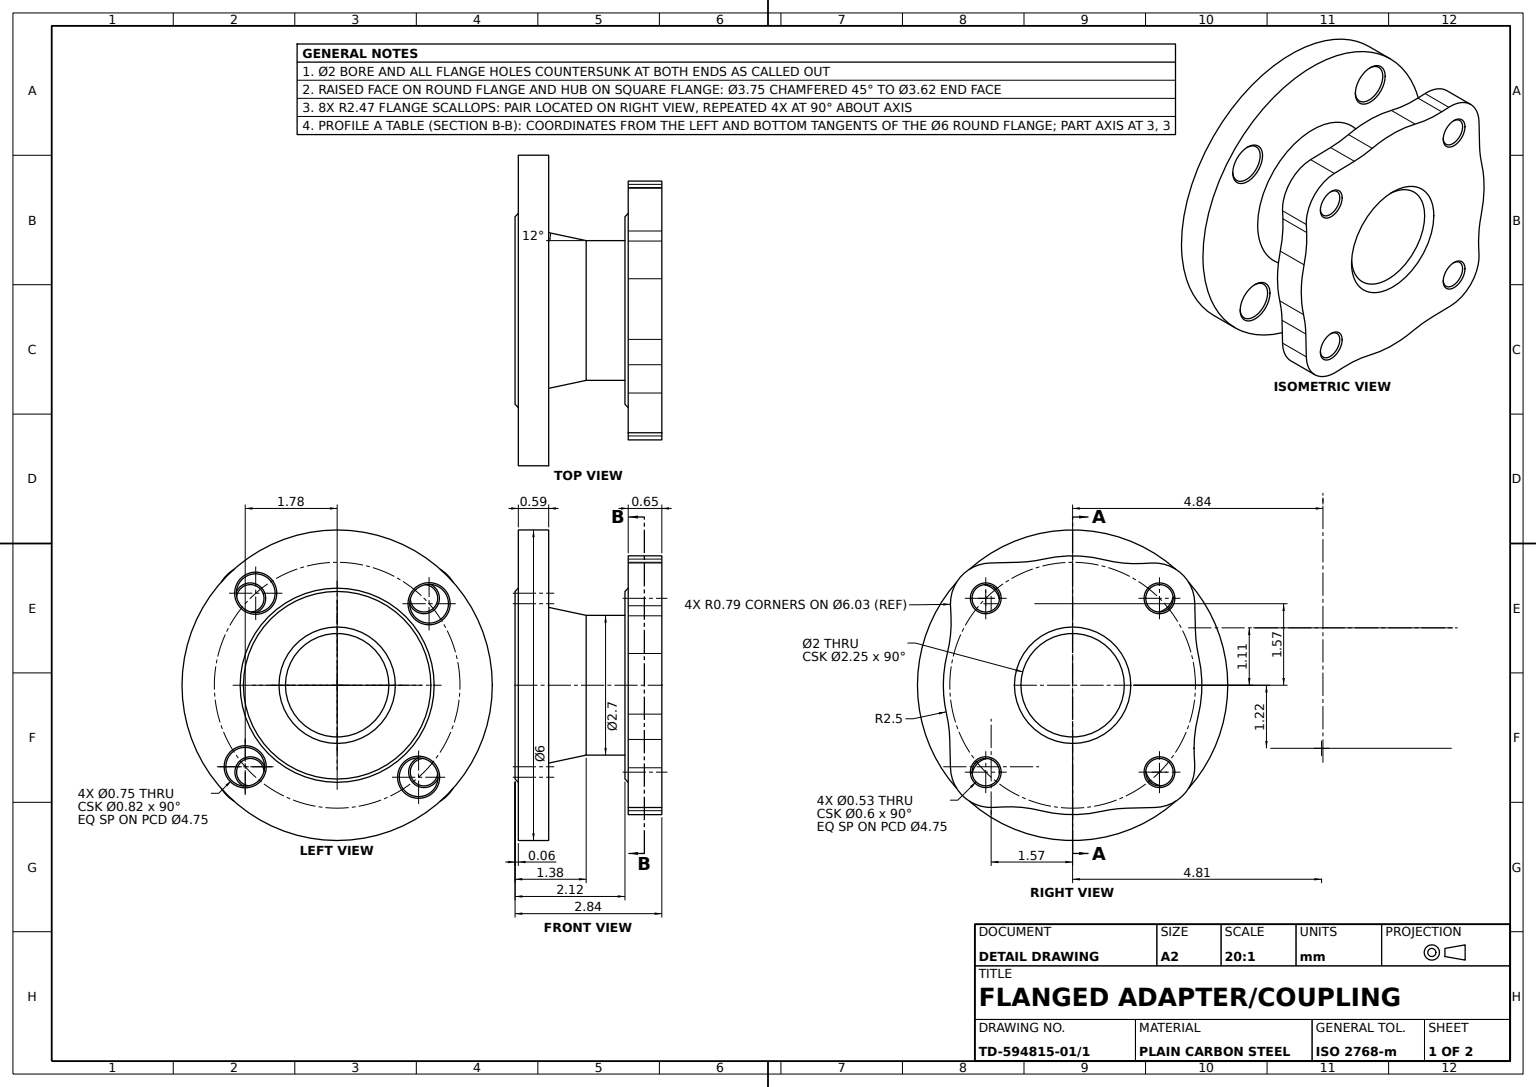
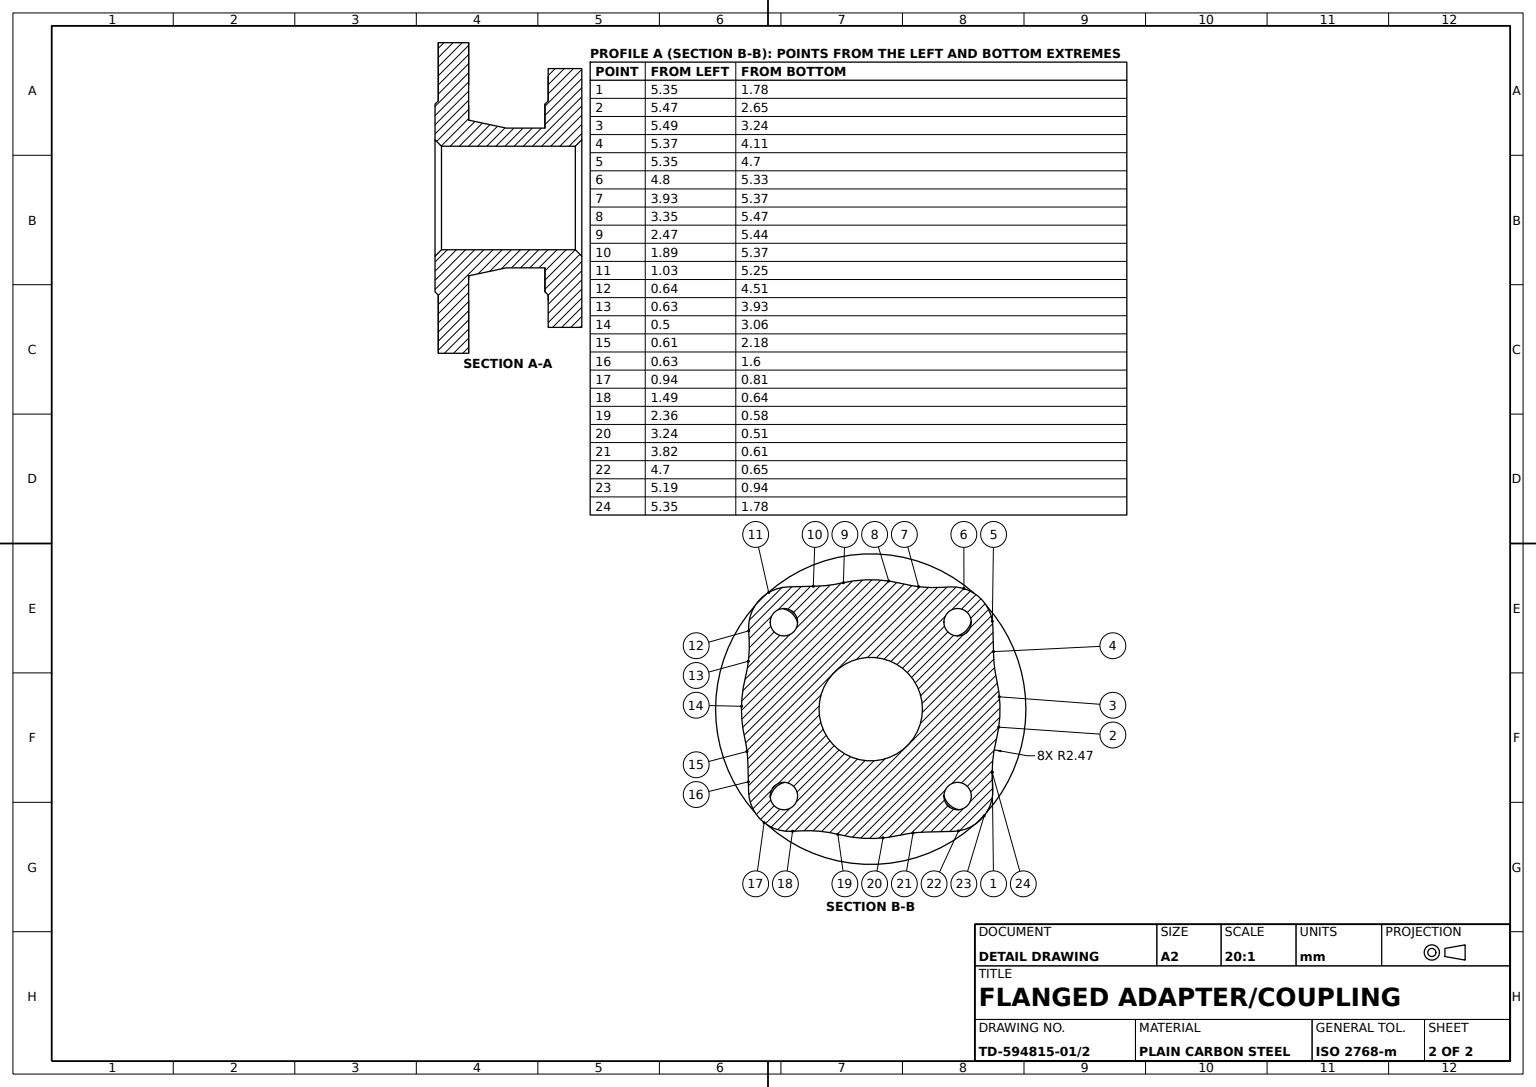
SolidWorks part; units mm, degrees
material "Plain Carbon Steel"
ref_plane "Front Plane" through (0, 0, 0) normal (0, 0, 1) x (1, 0, 0)
ref_plane "Top Plane" through (0, 0, 0) normal (0, 1, 0) x (1, 0, 0)
ref_plane "Right Plane" through (0, 0, 0) normal (1, 0, 0) x (0, 0, -1)
sketch "Housing Profile Sketch" plane through (0, 0, 0) normal (0, 0, 1) x (1, 0, 0)
  line L0 (0, 1) -> (0, 1.8125)
  line L1 (0, 1.8125) -> (0.063, 1.8755)
  line L2 (0.063, 1.8755) -> (0.063, 3)
  line L3 (0.063, 3) -> (0.65, 3)
  line L4 (0.65, 3) -> (0.65, 1.5041)
  line L5 (0.65, 1.5041) -> (1.375, 1.35)
  line L6 (1.375, 1.35) -> (2.125, 1.35)
  line L7 (2.125, 1.35) -> (2.125, 1.812)
  line L8 (2.125, 1.812) -> (2.188, 1.875)
  line L12 (2.188, 1) -> (0, 1)
  line L13 (0, 0) -> (6.1137, 0) construction
  line L14 (2.188, 1.875) -> (2.188, 1)
  dimension "D1" = 1.8125
  dimension "D2" = 3
  dimension "D3" = 45
  dimension "D4" = 0.65
  dimension "D5" = 0.063
  dimension "D7" = 1.375
  dimension "D8" = 2.125
  dimension "D9" = 1
  dimension "D10" = 1.35
  dimension "D11" = 1.875
  dimension "D13" = 12
  dimension "D14" = 0.063
revolve "Housing Body Revolve" add sketch "Housing Profile Sketch" angle 360 about L13
sketch "Square Flange Sketch" plane through (2.188, 0, 0) normal (1, 0, 0) x (0, 0, -1)
  line L0 (0, 0) -> (0, 2.5498) construction
  line L1 (0, 0) -> (-2.4311, 2.4311) construction
  line L2 (-1.5946, 2.3618) -> (-1.0477, 2.3753)
  line L3 (-2.361, 1.5357) -> (-2.3513, 1.3414)
  line L4 (1.5357, 2.361) -> (1.3414, 2.3513)
  line L5 (2.3618, 1.5946) -> (2.3753, 1.0477)
  line L6 (2.361, -1.5357) -> (2.3513, -1.3414)
  line L7 (1.5946, -2.3618) -> (1.0477, -2.3753)
  line L8 (-1.5357, -2.361) -> (-1.3414, -2.3513)
  line L9 (-2.3618, -1.5946) -> (-2.3753, -1.0477)
  arc A2 (-1.5946, 2.3618) -> (-2.361, 1.5357) centre (-1.575, 1.575) ccw
  circle A7 centre (0, 0) radius 2.375 construction
  circle A8 centre (0, 0) radius 1 construction
  circle A9 centre (0, 0) radius 1
  arc A10 (-2.4236, 0.6134) -> (-2.4369, -0.5583) centre (0, 0) ccw
  arc A12 (2.3618, 1.5946) -> (1.5357, 2.361) centre (1.575, 1.575) ccw
  arc A14 (-2.3618, -1.5946) -> (-1.5357, -2.361) centre (-1.575, -1.575) ccw
  arc A15 (0.6134, 2.4236) -> (-0.5583, 2.4369) centre (0, 0) ccw
  arc A16 (-0.6134, -2.4236) -> (0.5583, -2.4369) centre (0, 0) ccw
  arc A17 (2.4236, -0.6134) -> (2.4369, 0.5583) centre (0, 0) ccw
  arc A18 (1.5946, -2.3618) -> (2.361, -1.5357) centre (1.575, -1.575) ccw
  circle A19 centre (-1.6794, 1.6794) radius 0.265
  circle A20 centre (1.6794, 1.6794) radius 0.265
  circle A21 centre (1.6794, -1.6794) radius 0.265
  circle A22 centre (-1.6794, -1.6794) radius 0.265
  arc A23 (-0.5583, 2.4369) -> (-1.0477, 2.3753) centre (-1.109, 4.8404) cw
  arc A24 (1.3414, 2.3513) -> (0.6134, 2.4236) centre (1.2183, 4.814) cw
  arc A25 (2.3753, 1.0477) -> (2.4369, 0.5583) centre (4.8404, 1.109) ccw
  arc A26 (2.3513, -1.3414) -> (2.4236, -0.6134) centre (4.814, -1.2183) cw
  arc A27 (1.0477, -2.3753) -> (0.5583, -2.4369) centre (1.109, -4.8404) ccw
  arc A28 (-1.3414, -2.3513) -> (-0.6134, -2.4236) centre (-1.2183, -4.814) cw
  arc A29 (-2.3753, -1.0477) -> (-2.4369, -0.5583) centre (-4.8404, -1.109) ccw
  arc A30 (-2.3513, 1.3414) -> (-2.4236, 0.6134) centre (-4.814, 1.2183) cw
  circle A31 centre (0, 0) radius 1.875 construction
  point P16 (0, 0)
  point P24 (0, 0)
  point P37 (0, 0)
  point P43 (0, 0)
  dimension "D1" = 45
  dimension "D2" = 4.75
  dimension "D3" = 5
  dimension "D4" = 4
  dimension "D6" = 0.53
  dimension "D8" = 2.4658
  dimension "D9" = 0.787
  dimension "D5" = 1.575
  dimension "D7" = 4
  dimension "D10" = 0.5583
  dimension "D11" = 0.6134
extrude "Square Outlet Flange" add sketch "Square Flange Sketch" along normal blind 0.65
sketch "Round Flange Holes Sketch" plane through (0.063, 0, 0) normal (-1, 0, 0) x (0, 0, 1)
  circle A1 centre (0, 0) radius 2.375 construction
  circle A2 centre (-1.575, 1.7776) radius 0.375
  circle A3 centre (1.7776, 1.575) radius 0.375
  circle A4 centre (1.575, -1.7776) radius 0.375
  circle A5 centre (-1.7776, -1.575) radius 0.375
  point P15 (0, 0)
  dimension "D1" = 4.75
  dimension "D2" = 0.75
  dimension "D3" = 1.575
  dimension "D4" = 4
extrude "Round Flange Holes 4xØ0.75" cut sketch "Round Flange Holes Sketch" against normal blind 0.65
chamfer "Round Flange Hole Chamfers" distance 0.0325 angle 45 8 edges at (0.65, -1.575, -1.4026) (0.063, -1.575, -1.4026) (0.65, -1.7776, 1.95) (0.063, -1.7776, 1.95) (0.65, 1.575, 2.1526) (0.063, 1.575, 2.1526) (0.65, 1.7776, -1.2) (0.063, 1.7776, -1.2)
chamfer "Square Flange Chamfers" distance 0.0325 angle 45 8 edges at (2.188, -1.6794, 1.4144) (2.838, -1.6794, 1.4144) (2.188, -1.6794, -1.9444) (2.838, -1.6794, -1.9444) (2.188, 1.6794, -1.9444) (2.838, 1.6794, -1.9444) (2.188, 1.6794, 1.4144) (2.838, 1.6794, 1.4144)
chamfer "Housing Edge Chamfers" distance 0.125 angle 45 2 edges at (2.838, 0, -1) (0, 0, 1)
